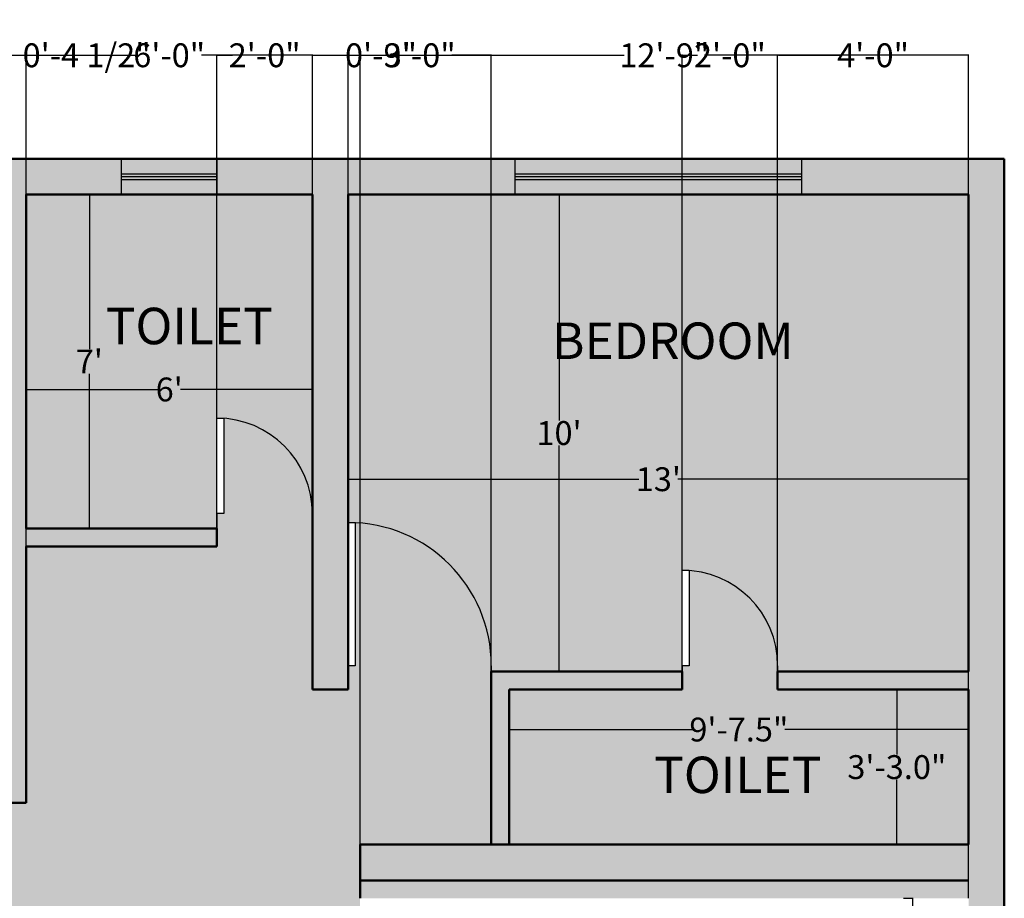
# Model space of a CAD drawing. Units: inches. Extents: x 1379 to 6665, y -118 to 1026.
# Tile 11 of 29: x 2532 to 2779, y 426 to 647. Entities that reach past the tile are written whole.
import ezdxf

# ---------------------------------------------------------------- set-up
doc = ezdxf.new("R2010")
doc.units = ezdxf.units.IN
doc.header["$MEASUREMENT"] = 0
for name, color, linetype, lineweight in [('A-ANNO-DIMS', 2, 'Continuous', 18), ('A-AREA-IDEN', 7, 'Continuous', 25), ('A-DOOR', 1, 'Continuous', 25), ('A-FLOR-PATT', 252, 'Continuous', 13), ('A-GLAZ', 2, 'Continuous', 25), ('A-WALL', 7, 'Continuous', 50), ('A-WALL-PATT', 8, 'Continuous', 13)]:
    doc.layers.add(name, color=color, linetype=linetype, lineweight=lineweight)
doc.styles.get("Standard").update_dxf_attribs({"font": 'arial.ttf'})
doc.dimstyles.get("Standard").update_dxf_attribs({"dimtxt": 6, "dimasz": 0.18, "dimexe": 0.18, "dimexo": 0.0625, "dimgap": 0.09, "dimtad": 0, "dimtih": 1, "dimtoh": 1, "dimdec": 1, "dimzin": 0, "dimdsep": 46, "dimlunit": 3, "dimtxsty": 'Standard', "dimcen": 0.09, "dimclrt": 250, "dimadec": 0, "dimazin": 0, "dimtfac": 1, "dimtdec": 1, "dimtofl": 0, "dimtmove": 0, "dimatfit": 3, "dimfxl": 1, "dimtolj": 1, "dimtzin": 0, "dimarcsym": 0})

# ---------------------------------------------------------------- blocks, each defined once
blk = doc.blocks.new('*D24')
at = {"layer": 'A-ANNO-DIMS', "color": 0, "lineweight": -2, "transparency": 16777216}
for p, q in [((2753.97, 425.93), (2756.45, 425.93)), ((2756.27, 425.75), (2756.27, 387.02)), ((2756.27, 342.11), (2756.27, 380.84)), ((2753.97, 341.93), (2756.45, 341.93))]:
    blk.add_line(p, q, dxfattribs=at)
at = {"layer": 'A-ANNO-DIMS', "color": 0, "transparency": 16777216}
for points in [[(2756.24, 425.75), (2756.3, 425.75), (2756.27, 425.93)], [(2756.24, 342.11), (2756.3, 342.11), (2756.27, 341.93)]]:
    blk.add_solid(points, dxfattribs=at)
at = {"layer": 'Defpoints', "color": 0, "transparency": 16777216}
for p in [(2753.9, 425.93), (2753.9, 341.93), (2756.27, 341.93)]:
    blk.add_point(p, dxfattribs=at)
at = {"layer": 'A-ANNO-DIMS', "color": 0, "transparency": 16777216, "insert": (2756.27, 383.93), "char_height": 6, "attachment_point": 5}
blk.add_mtext("\\A1;7'", dxfattribs=at)
blk = doc.blocks.new('*U2')
for p, q in [((0, 0), (0, -6)), ((24, 0), (24, -6))]:
    blk.add_line(p, q)
blk.add_lwpolyline([(0, 0), (0, 24), (1.75, 24), (1.75, 0)], close=True)
blk.add_arc((0, 0), 24, 0, 90)
blk = doc.blocks.new('*U3')
for p, q in [((0, 0), (0, -6)), ((36, 0), (36, -6))]:
    blk.add_line(p, q)
blk.add_lwpolyline([(0, 0), (0, 36), (1.75, 36), (1.75, 0)], close=True)
blk.add_arc((0, 0), 36, 0, 90)
blk = doc.blocks.new('*D30')
at = {"layer": 'A-ANNO-DIMS', "color": 0, "lineweight": -2, "transparency": 16777216}
for p, q in [((2533.35, 553.83), (2533.35, 553.71)), ((2533.53, 553.89), (2566.48, 553.89)), ((2605.17, 553.89), (2572.22, 553.89)), ((2605.35, 553.95), (2605.35, 554.07))]:
    blk.add_line(p, q, dxfattribs=at)
at = {"layer": 'A-ANNO-DIMS', "color": 0, "transparency": 16777216}
for points in [[(2533.53, 553.92), (2533.53, 553.86), (2533.35, 553.89)], [(2605.17, 553.92), (2605.17, 553.86), (2605.35, 553.89)]]:
    blk.add_solid(points, dxfattribs=at)
at = {"layer": 'Defpoints', "color": 0, "transparency": 16777216}
for p in [(2533.35, 553.89), (2605.35, 553.89), (2605.35, 553.89)]:
    blk.add_point(p, dxfattribs=at)
at = {"layer": 'A-ANNO-DIMS', "color": 0, "transparency": 16777216, "insert": (2569.35, 553.89), "char_height": 6, "attachment_point": 5}
blk.add_mtext("\\A1;6'", dxfattribs=at)
blk = doc.blocks.new('*D31')
at = {"layer": 'A-ANNO-DIMS', "color": 0, "lineweight": -2, "transparency": 16777216}
for p, q in [((2546.25, 602.93), (2549.44, 602.93)), ((2549.26, 602.75), (2549.26, 564.02)), ((2549.26, 519.11), (2549.26, 557.84)), ((2546.25, 518.93), (2549.44, 518.93))]:
    blk.add_line(p, q, dxfattribs=at)
at = {"layer": 'A-ANNO-DIMS', "color": 0, "transparency": 16777216}
for points in [[(2549.23, 602.75), (2549.29, 602.75), (2549.26, 602.93)], [(2549.23, 519.11), (2549.29, 519.11), (2549.26, 518.93)]]:
    blk.add_solid(points, dxfattribs=at)
at = {"layer": 'Defpoints', "color": 0, "transparency": 16777216}
for p in [(2546.19, 602.93), (2546.19, 518.93), (2549.26, 518.93)]:
    blk.add_point(p, dxfattribs=at)
at = {"layer": 'A-ANNO-DIMS', "color": 0, "transparency": 16777216, "insert": (2549.26, 560.93), "char_height": 6, "attachment_point": 5}
blk.add_mtext("\\A1;7'", dxfattribs=at)
blk = doc.blocks.new('*D32')
at = {"layer": 'A-ANNO-DIMS', "color": 0, "lineweight": -2, "transparency": 16777216}
for p, q in [((2649.05, 602.93), (2667.55, 602.93)), ((2667.37, 602.75), (2667.37, 546.09)), ((2667.37, 483.11), (2667.37, 539.78)), ((2663.46, 482.93), (2667.55, 482.93))]:
    blk.add_line(p, q, dxfattribs=at)
at = {"layer": 'A-ANNO-DIMS', "color": 0, "transparency": 16777216}
for points in [[(2667.34, 602.75), (2667.4, 602.75), (2667.37, 602.93)], [(2667.34, 483.11), (2667.4, 483.11), (2667.37, 482.93)]]:
    blk.add_solid(points, dxfattribs=at)
at = {"layer": 'Defpoints', "color": 0, "transparency": 16777216}
for p in [(2648.99, 602.93), (2663.4, 482.93), (2667.37, 482.93)]:
    blk.add_point(p, dxfattribs=at)
at = {"layer": 'A-ANNO-DIMS', "color": 0, "transparency": 16777216, "insert": (2667.37, 542.93), "char_height": 6, "attachment_point": 5}
blk.add_mtext("\\A1;10'", dxfattribs=at)
blk = doc.blocks.new('*D33')
at = {"layer": 'A-ANNO-DIMS', "color": 0, "lineweight": -2, "transparency": 16777216}
for p, q in [((2614.35, 529.56), (2614.35, 531.5)), ((2614.53, 531.32), (2687.45, 531.32)), ((2770.17, 531.32), (2697.25, 531.32)), ((2770.35, 527.24), (2770.35, 531.5))]:
    blk.add_line(p, q, dxfattribs=at)
at = {"layer": 'A-ANNO-DIMS', "color": 0, "transparency": 16777216}
for points in [[(2614.53, 531.35), (2614.53, 531.29), (2614.35, 531.32)], [(2770.17, 531.35), (2770.17, 531.29), (2770.35, 531.32)]]:
    blk.add_solid(points, dxfattribs=at)
at = {"layer": 'Defpoints', "color": 0, "transparency": 16777216}
for p in [(2770.35, 531.32), (2614.35, 529.5), (2770.35, 527.18)]:
    blk.add_point(p, dxfattribs=at)
at = {"layer": 'A-ANNO-DIMS', "color": 0, "transparency": 16777216, "insert": (2692.35, 531.32), "char_height": 6, "attachment_point": 5}
blk.add_mtext("\\A1;13'", dxfattribs=at)
blk = doc.blocks.new('*D34')
at = {"layer": 'A-ANNO-DIMS', "color": 0, "lineweight": -2, "transparency": 16777216}
for p, q in [((2751.31, 478.43), (2752.51, 478.43)), ((2752.33, 478.25), (2752.33, 462.09)), ((2752.33, 439.61), (2752.33, 455.78)), ((2751.31, 439.43), (2752.51, 439.43))]:
    blk.add_line(p, q, dxfattribs=at)
at = {"layer": 'A-ANNO-DIMS', "color": 0, "transparency": 16777216}
for points in [[(2752.3, 478.25), (2752.36, 478.25), (2752.33, 478.43)], [(2752.3, 439.61), (2752.36, 439.61), (2752.33, 439.43)]]:
    blk.add_solid(points, dxfattribs=at)
at = {"layer": 'Defpoints', "color": 0, "transparency": 16777216}
for p in [(2751.25, 478.43), (2751.25, 439.43), (2752.33, 439.43)]:
    blk.add_point(p, dxfattribs=at)
at = {"layer": 'A-ANNO-DIMS', "color": 0, "transparency": 16777216, "insert": (2752.33, 458.93), "char_height": 6, "attachment_point": 5}
blk.add_mtext('\\A1;3\'-3.0"', dxfattribs=at)
blk = doc.blocks.new('*D35')
at = {"layer": 'A-ANNO-DIMS', "color": 0, "lineweight": -2, "transparency": 16777216}
for p, q in [((2654.85, 463.04), (2654.85, 468.56)), ((2655.03, 468.38), (2701.04, 468.38)), ((2770.17, 468.38), (2724.16, 468.38)), ((2770.35, 459), (2770.35, 468.56))]:
    blk.add_line(p, q, dxfattribs=at)
at = {"layer": 'A-ANNO-DIMS', "color": 0, "transparency": 16777216}
for points in [[(2655.03, 468.41), (2655.03, 468.35), (2654.85, 468.38)], [(2770.17, 468.41), (2770.17, 468.35), (2770.35, 468.38)]]:
    blk.add_solid(points, dxfattribs=at)
at = {"layer": 'Defpoints', "color": 0, "transparency": 16777216}
for p in [(2770.35, 468.38), (2654.85, 462.97), (2770.35, 458.93)]:
    blk.add_point(p, dxfattribs=at)
at = {"layer": 'A-ANNO-DIMS', "color": 0, "transparency": 16777216, "insert": (2712.6, 468.38), "char_height": 6, "attachment_point": 5}
blk.add_mtext('\\A1;9\'-7.5"', dxfattribs=at)
blk = doc.blocks.new('WIN-1800')
for p, q in [((0, 0.73), (72, 0.73)), ((0, 0), (72, 0))]:
    blk.add_line(p, q)
blk = doc.blocks.new('WIN-600')
for p, q in [((0, 24), (0, 0)), ((0.73, 24), (0.73, 0))]:
    blk.add_line(p, q)
blk = doc.blocks.new('*D155')
at = {"layer": 'A-ANNO-DIMS', "color": 0, "lineweight": -2, "transparency": 16777216}
for p, q in [((2528.85, 603), (2528.85, 638.11)), ((2529.03, 637.93), (2533.17, 637.93)), ((2533.35, 603), (2533.35, 638.11)), ((2533.35, 637.93), (2533.53, 637.93))]:
    blk.add_line(p, q, dxfattribs=at)
at = {"layer": 'A-ANNO-DIMS', "color": 0, "transparency": 16777216}
for points in [[(2529.03, 637.96), (2529.03, 637.9), (2528.85, 637.93)], [(2533.17, 637.96), (2533.17, 637.9), (2533.35, 637.93)]]:
    blk.add_solid(points, dxfattribs=at)
at = {"layer": 'Defpoints', "color": 0, "transparency": 16777216}
for p in [(2533.35, 637.93), (2528.85, 602.93), (2533.35, 602.93)]:
    blk.add_point(p, dxfattribs=at)
at = {"layer": 'A-ANNO-DIMS', "color": 250, "transparency": 16777216, "insert": (2548.59, 637.93), "char_height": 6, "attachment_point": 5}
blk.add_mtext('\\A1;0\'-4 1/2"', dxfattribs=at)
blk = doc.blocks.new('*D156')
at = {"layer": 'A-ANNO-DIMS', "color": 0, "lineweight": -2, "transparency": 16777216}
for p, q in [((2605.35, 603), (2605.35, 638.11)), ((2605.53, 637.93), (2614.17, 637.93)), ((2614.35, 603), (2614.35, 638.11)), ((2614.35, 637.93), (2614.53, 637.93))]:
    blk.add_line(p, q, dxfattribs=at)
at = {"layer": 'A-ANNO-DIMS', "color": 0, "transparency": 16777216}
for points in [[(2605.53, 637.96), (2605.53, 637.9), (2605.35, 637.93)], [(2614.17, 637.96), (2614.17, 637.9), (2614.35, 637.93)]]:
    blk.add_solid(points, dxfattribs=at)
at = {"layer": 'Defpoints', "color": 0, "transparency": 16777216}
for p in [(2614.35, 637.93), (2605.35, 602.93), (2614.35, 602.93)]:
    blk.add_point(p, dxfattribs=at)
at = {"layer": 'A-ANNO-DIMS', "color": 250, "transparency": 16777216, "insert": (2622.6, 637.93), "char_height": 6, "attachment_point": 5}
blk.add_mtext('\\A1;0\'-9"', dxfattribs=at)
blk = doc.blocks.new('*D157')
at = {"layer": 'A-ANNO-DIMS', "color": 0, "lineweight": -2, "transparency": 16777216}
for p, q in [((2533.35, 514.5), (2533.35, 638.11)), ((2533.53, 637.93), (2561.27, 637.93)), ((2605.17, 637.93), (2577.43, 637.93)), ((2605.35, 478.5), (2605.35, 638.11))]:
    blk.add_line(p, q, dxfattribs=at)
at = {"layer": 'A-ANNO-DIMS', "color": 0, "transparency": 16777216}
for points in [[(2533.53, 637.96), (2533.53, 637.9), (2533.35, 637.93)], [(2605.17, 637.96), (2605.17, 637.9), (2605.35, 637.93)]]:
    blk.add_solid(points, dxfattribs=at)
at = {"layer": 'Defpoints', "color": 0, "transparency": 16777216}
for p in [(2605.35, 637.93), (2533.35, 514.43), (2605.35, 478.43)]:
    blk.add_point(p, dxfattribs=at)
at = {"layer": 'A-ANNO-DIMS', "color": 250, "transparency": 16777216, "insert": (2569.35, 637.93), "char_height": 6, "attachment_point": 5}
blk.add_mtext('\\A1;6\'-0"', dxfattribs=at)
blk = doc.blocks.new('*D158')
at = {"layer": 'A-ANNO-DIMS', "color": 0, "lineweight": -2, "transparency": 16777216}
for p, q in [((2617.35, 426), (2617.35, 638.11)), ((2617.53, 637.93), (2683.74, 637.93)), ((2770.17, 637.93), (2703.96, 637.93)), ((2770.35, 426), (2770.35, 638.11))]:
    blk.add_line(p, q, dxfattribs=at)
at = {"layer": 'A-ANNO-DIMS', "color": 0, "transparency": 16777216}
for points in [[(2617.53, 637.96), (2617.53, 637.9), (2617.35, 637.93)], [(2770.17, 637.96), (2770.17, 637.9), (2770.35, 637.93)]]:
    blk.add_solid(points, dxfattribs=at)
at = {"layer": 'Defpoints', "color": 0, "transparency": 16777216}
for p in [(2770.35, 637.93), (2617.35, 425.93), (2770.35, 425.93)]:
    blk.add_point(p, dxfattribs=at)
at = {"layer": 'A-ANNO-DIMS', "color": 250, "transparency": 16777216, "insert": (2693.85, 637.93), "char_height": 6, "attachment_point": 5}
blk.add_mtext('\\A1;12\'-9"', dxfattribs=at)
blk = doc.blocks.new('*D162')
at = {"layer": 'A-ANNO-DIMS', "color": 0, "lineweight": -2, "transparency": 16777216}
for p, q in [((2581.35, 519), (2581.35, 638.11)), ((2581.53, 637.93), (2585.23, 637.93)), ((2605.17, 637.93), (2601.47, 637.93)), ((2605.35, 519), (2605.35, 638.11))]:
    blk.add_line(p, q, dxfattribs=at)
at = {"layer": 'A-ANNO-DIMS', "color": 0, "transparency": 16777216}
for points in [[(2581.53, 637.96), (2581.53, 637.9), (2581.35, 637.93)], [(2605.17, 637.96), (2605.17, 637.9), (2605.35, 637.93)]]:
    blk.add_solid(points, dxfattribs=at)
at = {"layer": 'Defpoints', "color": 0, "transparency": 16777216}
for p in [(2605.35, 637.93), (2581.35, 518.93), (2605.35, 518.93)]:
    blk.add_point(p, dxfattribs=at)
at = {"layer": 'A-ANNO-DIMS', "color": 250, "transparency": 16777216, "insert": (2593.35, 637.93), "char_height": 6, "attachment_point": 5}
blk.add_mtext('\\A1;2\'-0"', dxfattribs=at)
blk = doc.blocks.new('*D164')
at = {"layer": 'A-ANNO-DIMS', "color": 0, "lineweight": -2, "transparency": 16777216}
for p, q in [((2614.35, 483), (2614.35, 638.11)), ((2614.53, 637.93), (2624.29, 637.93)), ((2650.17, 637.93), (2640.41, 637.93)), ((2650.35, 483), (2650.35, 638.11))]:
    blk.add_line(p, q, dxfattribs=at)
at = {"layer": 'A-ANNO-DIMS', "color": 0, "transparency": 16777216}
for points in [[(2614.53, 637.96), (2614.53, 637.9), (2614.35, 637.93)], [(2650.17, 637.96), (2650.17, 637.9), (2650.35, 637.93)]]:
    blk.add_solid(points, dxfattribs=at)
at = {"layer": 'Defpoints', "color": 0, "transparency": 16777216}
for p in [(2650.35, 637.93), (2614.35, 482.93), (2650.35, 482.93)]:
    blk.add_point(p, dxfattribs=at)
at = {"layer": 'A-ANNO-DIMS', "color": 250, "transparency": 16777216, "insert": (2632.35, 637.93), "char_height": 6, "attachment_point": 5}
blk.add_mtext('\\A1;3\'-0"', dxfattribs=at)
blk = doc.blocks.new('*D166')
at = {"layer": 'A-ANNO-DIMS', "color": 0, "lineweight": -2, "transparency": 16777216}
for p, q in [((2698.35, 483), (2698.35, 638.11)), ((2698.53, 637.93), (2702.23, 637.93)), ((2722.17, 637.93), (2718.47, 637.93)), ((2722.35, 483), (2722.35, 638.11))]:
    blk.add_line(p, q, dxfattribs=at)
at = {"layer": 'A-ANNO-DIMS', "color": 0, "transparency": 16777216}
for points in [[(2698.53, 637.96), (2698.53, 637.9), (2698.35, 637.93)], [(2722.17, 637.96), (2722.17, 637.9), (2722.35, 637.93)]]:
    blk.add_solid(points, dxfattribs=at)
at = {"layer": 'Defpoints', "color": 0, "transparency": 16777216}
for p in [(2722.35, 637.93), (2698.35, 482.93), (2722.35, 482.93)]:
    blk.add_point(p, dxfattribs=at)
at = {"layer": 'A-ANNO-DIMS', "color": 250, "transparency": 16777216, "insert": (2710.35, 637.93), "char_height": 6, "attachment_point": 5}
blk.add_mtext('\\A1;2\'-0"', dxfattribs=at)
blk = doc.blocks.new('*D167')
at = {"layer": 'A-ANNO-DIMS', "color": 0, "lineweight": -2, "transparency": 16777216}
for p, q in [((2722.35, 483), (2722.35, 638.11)), ((2722.53, 637.93), (2738.16, 637.93)), ((2770.17, 637.93), (2754.54, 637.93)), ((2770.35, 483), (2770.35, 638.11))]:
    blk.add_line(p, q, dxfattribs=at)
at = {"layer": 'A-ANNO-DIMS', "color": 0, "transparency": 16777216}
for points in [[(2722.53, 637.96), (2722.53, 637.9), (2722.35, 637.93)], [(2770.17, 637.96), (2770.17, 637.9), (2770.35, 637.93)]]:
    blk.add_solid(points, dxfattribs=at)
at = {"layer": 'Defpoints', "color": 0, "transparency": 16777216}
for p in [(2770.35, 637.93), (2722.35, 482.93), (2770.35, 482.93)]:
    blk.add_point(p, dxfattribs=at)
at = {"layer": 'A-ANNO-DIMS', "color": 250, "transparency": 16777216, "insert": (2746.35, 637.93), "char_height": 6, "attachment_point": 5}
blk.add_mtext('\\A1;4\'-0"', dxfattribs=at)

msp = doc.modelspace()

# ---------------------------------------------------------------- hatches: boundary and pattern name
at = {"layer": 'A-FLOR-PATT', "transparency": 33554590}
h = msp.add_hatch(color=256, dxfattribs=at)
h.dxf.hatch_style = 1
h.paths.add_polyline_path([(2290.35, 490.43), (2290.35, 602.93), (2369.85, 602.93), (2369.85, 611.93), (2281.35, 611.93), (2281.35, 499.43), (2281.35, 431.93), (2290.35, 431.93), (2290.35, 449.93), (2462.85, 449.93), (2462.85, 458.93), (2290.35, 458.93)])
h.paths.add_polyline_path([(2462.85, 341.93), (2290.35, 341.93), (2290.35, 359.93), (2281.35, 359.93), (2281.35, 179.93), (2359.96, 179.93), (2359.96, 188.93), (2290.35, 188.93), (2290.35, 332.93), (2462.85, 332.93)])
h.paths.add_polyline_path([(2557.35, 188.93), (2533.35, 188.93), (2533.35, 272.93), (2581.35, 272.93), (2581.35, 277.43), (2533.35, 277.43), (2533.35, 332.93), (2533.35, 341.93), (2498.82, 341.93), (2498.85, 332.93), (2528.85, 332.93), (2528.85, 188.93), (2431.96, 188.93), (2431.96, 179.93), (2557.35, 179.93)])
h.paths.add_polyline_path([(2666.85, 188.93), (2614.35, 188.93), (2614.35, 277.43), (2605.35, 277.43), (2605.35, 272.93), (2605.35, 188.93), (2581.35, 188.93), (2581.35, 179.93), (2617.35, 179.93), (2666.85, 179.93)])
h.paths.add_polyline_path([(2779.35, 296.93), (2770.35, 296.93), (2770.35, 284.93), (2740.35, 284.93), (2740.35, 280.43), (2770.35, 280.43), (2770.35, 188.93), (2738.85, 188.93), (2738.85, 179.93), (2779.35, 179.93)])
h.paths.add_polyline_path([(2779.35, 611.93), (2728.35, 611.93), (2728.35, 602.93), (2770.35, 602.93), (2770.35, 482.93), (2722.35, 482.93), (2722.35, 478.43), (2770.35, 478.43), (2770.35, 439.43), (2626.35, 439.43), (2617.35, 439.43), (2617.35, 430.43), (2617.35, 425.93), (2770.35, 425.93), (2770.35, 341.93), (2617.35, 341.93), (2569.35, 341.93), (2569.35, 332.93), (2617.35, 332.93), (2681.85, 332.93), (2681.85, 284.93), (2654.35, 284.93), (2654.35, 280.43), (2681.85, 280.43), (2716.35, 280.43), (2716.35, 284.93), (2686.35, 284.93), (2686.35, 332.93), (2770.35, 332.93), (2770.35, 320.93), (2779.35, 320.93)])
h.paths.add_polyline_path([(2698.35, 482.93), (2650.35, 482.93), (2650.35, 478.43), (2650.35, 439.43), (2654.85, 439.43), (2654.85, 478.43), (2698.35, 478.43)], flags=17)
h.paths.add_polyline_path([(2614.35, 602.93), (2656.35, 602.93), (2656.35, 611.93), (2581.35, 611.93), (2581.35, 602.93), (2605.35, 602.93), (2605.35, 478.43), (2614.35, 478.43), (2614.35, 482.93)], flags=17)
h.paths.add_polyline_path([(2557.35, 611.93), (2521.35, 611.93), (2441.85, 611.93), (2441.85, 602.93), (2521.35, 602.93), (2528.85, 602.93), (2528.85, 458.93), (2498.73, 458.93), (2498.85, 449.93), (2533.35, 449.93), (2533.35, 514.43), (2581.35, 514.43), (2581.35, 518.93), (2533.35, 518.93), (2533.35, 602.93), (2557.35, 602.93)])
at = {"layer": 'A-WALL-PATT', "transparency": 33554590}
h = msp.add_hatch(color=256, dxfattribs=at)
h.dxf.hatch_style = 1
h.paths.add_polyline_path([(2581.35, 611.93), (2557.35, 611.93), (2557.35, 608.17), (2581.35, 608.17)])
h.paths.add_polyline_path([(2581.35, 606.7), (2557.35, 606.7), (2557.35, 602.93), (2581.35, 602.93)])
h.paths.add_polyline_path([(2581.35, 607.43), (2557.35, 607.43), (2557.35, 606.7), (2581.35, 606.7)])
h.paths.add_polyline_path([(2581.35, 608.17), (2557.35, 608.17), (2557.35, 607.43), (2581.35, 607.43)])
at = {"layer": 'A-WALL-PATT', "transparency": 33554564}
h = msp.add_hatch(color=256, dxfattribs=at)
h.dxf.hatch_style = 1
h.paths.add_polyline_path([(2728.35, 611.93), (2656.35, 611.93), (2656.35, 608.17), (2728.35, 608.17)])
h.paths.add_polyline_path([(2728.35, 607.43), (2656.35, 607.43), (2656.35, 606.7), (2728.35, 606.7)])
h.paths.add_polyline_path([(2728.35, 608.17), (2656.35, 608.17), (2656.35, 607.43), (2728.35, 607.43)])
h.paths.add_polyline_path([(2728.35, 606.7), (2656.35, 606.7), (2656.35, 602.93), (2728.35, 602.93)])
at = {"layer": 'A-WALL-PATT', "transparency": 33554590}
h = msp.add_hatch(color=256, dxfattribs=at)
h.dxf.hatch_style = 1
h.paths.add_polyline_path([(2528.85, 602.93), (2290.35, 602.93), (2290.35, 490.43), (2290.35, 458.93), (2462.85, 458.93), (2462.85, 491.93), (2464.6, 491.93), (2464.6, 491.89, -0.376042), (2498.73, 458.93), (2528.85, 458.93)])
h.paths.add_polyline_path([(2617.35, 425.93), (2617.35, 430.43), (2617.35, 439.43), (2626.35, 439.43), (2650.35, 439.43), (2650.35, 478.43), (2650.35, 484.43, 0.400041), (2616.1, 520.39), (2616.1, 484.43), (2614.35, 484.43), (2614.35, 478.43), (2605.35, 478.43), (2605.35, 522.68, 0.392996), (2583.1, 546.62), (2583.1, 522.68), (2581.35, 522.68), (2581.35, 516.68), (2581.35, 514.43), (2533.35, 514.43), (2533.35, 449.93), (2498.85, 449.93), (2498.73, 458.93, 0.376042), (2464.6, 491.89), (2464.6, 455.93), (2462.85, 455.93), (2462.85, 449.93), (2290.35, 449.93), (2290.35, 341.93), (2462.85, 341.93), (2462.85, 374.93), (2464.6, 374.93), (2464.6, 374.89, -0.376042), (2498.73, 341.93), (2533.35, 341.93), (2533.35, 332.93), (2533.35, 277.43), (2581.35, 277.43), (2581.35, 281.18), (2581.35, 305.18), (2583.1, 305.18), (2583.1, 305.12, -0.392996), (2605.35, 281.18), (2605.35, 277.43), (2614.35, 277.43), (2614.35, 283.43), (2614.35, 323.43), (2616.1, 323.43), (2616.1, 323.4, -0.390605), (2654.32, 284.93), (2681.85, 284.93), (2681.85, 332.93), (2614.35, 332.93), (2569.35, 332.93), (2569.35, 341.93), (2617.35, 341.93), (2617.35, 383.93)])
h.paths.add_polyline_path([(2605.35, 602.93), (2533.35, 602.93), (2533.35, 518.93), (2581.35, 518.93), (2581.35, 522.68), (2581.35, 546.68), (2583.1, 546.68), (2583.1, 546.62, -0.392996), (2605.35, 522.68)])
h.paths.add_polyline_path([(2770.35, 602.93), (2614.35, 602.93), (2614.35, 520.43), (2616.1, 520.43), (2616.1, 520.39, -0.400041), (2650.35, 484.43), (2650.35, 482.93), (2698.35, 482.93), (2698.35, 484.43), (2698.35, 508.43), (2700.1, 508.43), (2700.1, 508.37, -0.392996), (2722.35, 484.43), (2722.35, 482.93), (2770.35, 482.93)])
h.paths.add_polyline_path([(2528.85, 332.93), (2498.85, 332.93), (2498.82, 341.93), (2498.73, 341.93, 0.376042), (2464.6, 374.89), (2464.6, 374.93), (2462.85, 374.93), (2462.85, 341.93), (2462.85, 332.93), (2290.35, 332.93), (2290.35, 188.93), (2528.85, 188.93)])
h.paths.add_polyline_path([(2605.35, 272.93), (2605.35, 277.43), (2605.35, 281.18, 0.392996), (2583.1, 305.12), (2583.1, 281.18), (2581.35, 281.18), (2581.35, 277.43), (2581.35, 275.18), (2581.35, 272.93), (2533.35, 272.93), (2533.35, 188.93), (2605.35, 188.93)])
h.paths.add_polyline_path([(2770.35, 280.43), (2740.35, 280.43), (2740.35, 286.43, 0.392996), (2718.1, 310.37), (2718.1, 286.43), (2716.35, 286.43), (2716.35, 280.43), (2681.85, 280.43), (2654.35, 280.43), (2654.35, 283.43, 0.401453), (2616.1, 323.4), (2616.1, 283.43), (2614.35, 283.43), (2614.35, 277.43), (2614.35, 188.93), (2617.35, 188.93), (2770.35, 188.93)])
h.paths.add_polyline_path([(2770.35, 332.93), (2686.35, 332.93), (2686.35, 284.93), (2716.35, 284.93), (2716.35, 286.43), (2716.35, 310.43), (2718.1, 310.43), (2718.1, 310.37, -0.392996), (2740.35, 286.43), (2740.35, 284.93), (2770.35, 284.93)])
h.paths.add_polyline_path([(2770.35, 478.43), (2722.35, 478.43), (2722.35, 484.43, 0.392996), (2700.1, 508.37), (2700.1, 484.43), (2698.35, 484.43), (2698.35, 482.93), (2698.35, 478.43), (2654.85, 478.43), (2654.85, 439.43), (2770.35, 439.43)])
h.paths.add_polyline_path([(2372.98, 539.34), (2443.91, 539.34), (2443.91, 553.57), (2372.98, 553.57)], flags=24)
h.paths.add_polyline_path([(2370.72, 389.31), (2479.4, 389.31), (2479.4, 403.55), (2370.72, 403.55)], flags=24)
h.paths.add_polyline_path([(2550.99, 562.74), (2600.58, 562.74), (2600.58, 576.98), (2550.99, 576.98)], flags=24)
h.paths.add_polyline_path([(2663.19, 559.03), (2734.13, 559.03), (2734.13, 573.27), (2663.19, 573.27)], flags=24)
h.paths.add_polyline_path([(2372.98, 254.81), (2443.91, 254.81), (2443.91, 269.04), (2372.98, 269.04)], flags=24)
h.paths.add_polyline_path([(2545.25, 230.45), (2594.84, 230.45), (2594.84, 244.68), (2545.25, 244.68)], flags=24)
h.paths.add_polyline_path([(2664.48, 230.74), (2735.42, 230.74), (2735.42, 244.97), (2664.48, 244.97)], flags=24)
h.paths.add_polyline_path([(2704.72, 315.06), (2754.31, 315.06), (2754.31, 329.29), (2704.72, 329.29)], flags=24)
h.paths.add_polyline_path([(2688.89, 449.86), (2738.48, 449.86), (2738.48, 464.09), (2688.89, 464.09)], flags=24)

# ---------------------------------------------------------------- linework, layer by layer
at = {"layer": 'A-GLAZ'}
for p, q in [((2557.35, 606.7), (2581.35, 606.7)), ((2656.35, 606.7), (2728.35, 606.7))]:
    msp.add_line(p, q, dxfattribs=at)
for points in [[(2557.35, 611.93), (2581.35, 611.93), (2581.35, 602.93), (2557.35, 602.93)], [(2656.35, 611.93), (2728.35, 611.93), (2728.35, 602.93), (2656.35, 602.93)]]:
    msp.add_lwpolyline(points, close=True, dxfattribs=at)
at = {"layer": 'A-WALL'}
for p, q in [((2779.35, 611.93), (2521.35, 611.93)), ((2779.35, 611.93), (2779.35, 179.93)), ((2533.35, 518.93), (2533.35, 602.93)), ((2605.35, 602.93), (2533.35, 602.93)), ((2605.35, 478.43), (2605.35, 602.93)), ((2770.35, 602.93), (2614.35, 602.93)), ((2614.35, 482.93), (2614.35, 602.93)), ((2770.35, 602.93), (2770.35, 482.93)), ((2581.35, 518.93), (2533.35, 518.93)), ((2581.35, 518.93), (2581.35, 514.43)), ((2605.35, 518.93), (2605.35, 514.43)), ((2533.35, 449.93), (2533.35, 514.43)), ((2581.35, 514.43), (2533.35, 514.43)), ((2614.35, 482.93), (2614.35, 478.43)), ((2698.35, 482.93), (2650.35, 482.93)), ((2650.35, 482.93), (2650.35, 478.43)), ((2698.35, 478.43), (2698.35, 482.93)), ((2770.35, 482.93), (2722.35, 482.93)), ((2722.35, 478.43), (2722.35, 482.93)), ((2614.35, 478.43), (2605.35, 478.43)), ((2650.35, 478.43), (2650.35, 439.43)), ((2698.35, 478.43), (2654.85, 478.43)), ((2654.85, 478.43), (2654.85, 439.43)), ((2770.35, 478.43), (2722.35, 478.43)), ((2770.35, 478.43), (2770.35, 439.43)), ((2533.35, 449.93), (2498.85, 449.93)), ((2617.35, 430.43), (2617.35, 439.43)), ((2617.35, 439.43), (2626.35, 439.43)), ((2626.35, 439.43), (2770.35, 439.43)), ((2617.35, 430.43), (2617.35, 425.93)), ((2626.35, 430.43), (2617.35, 430.43)), ((2626.35, 430.43), (2770.35, 430.43))]:
    msp.add_line(p, q, dxfattribs=at)

# ---------------------------------------------------------------- block references
at = {"layer": 'A-DOOR'}
for name, p in [('*U2', (2581.35, 522.68)), ('*U3', (2614.35, 484.43)), ('*U2', (2698.35, 484.43))]:
    msp.add_blockref(name, p, dxfattribs=at)
at = {"layer": 'A-GLAZ', "rotation": 90.00000000000163}
msp.add_blockref('WIN-600', (2581.35, 607.43), dxfattribs=at)
at = {"layer": 'A-GLAZ'}
msp.add_blockref('WIN-1800', (2656.35, 607.43), dxfattribs=at)

# ---------------------------------------------------------------- texts
at = {"layer": 'A-AREA-IDEN'}
for s, p in [('TOILET', (2553.36, 565.27)), ('BEDROOM', (2665.56, 561.56)), ('TOILET', (2691.27, 452.39))]:
    msp.add_text(s, height=9.17, dxfattribs=at).set_placement(p)

# ---------------------------------------------------------------- dimensions: what is measured, and where the dimension line sits
at = {"layer": 'A-ANNO-DIMS'}
for base, p1, p2, override, picture, middle in [((2533.35, 637.93), (2528.85, 602.93), (2533.35, 602.93), {"dimdec": 1, "dimlfac": 1, "dimrnd": 0, "dimzin": 1, "dimdsep": 46, "dimlunit": 4, "dimfrac": 2}, '*D155', (2548.59, 637.93)), ((2605.35, 637.93), (2533.35, 514.43), (2605.35, 478.43), {"dimdec": 1, "dimlfac": 1, "dimrnd": 0, "dimzin": 1, "dimdsep": 46, "dimlunit": 4, "dimfrac": 2}, '*D157', (2569.35, 637.93)), ((2605.35, 637.93), (2581.35, 518.93), (2605.35, 518.93), {"dimdec": 1, "dimlfac": 1, "dimrnd": 0, "dimzin": 1, "dimdsep": 46, "dimlunit": 4, "dimfrac": 2}, '*D162', (2593.35, 637.93)), ((2614.35, 637.93), (2605.35, 602.93), (2614.35, 602.93), {"dimdec": 1, "dimlfac": 1, "dimrnd": 0, "dimzin": 1, "dimdsep": 46, "dimlunit": 4, "dimfrac": 2}, '*D156', (2622.6, 637.93)), ((2650.35, 637.93), (2614.35, 482.93), (2650.35, 482.93), {"dimdec": 1, "dimlfac": 1, "dimrnd": 0, "dimzin": 1, "dimdsep": 46, "dimlunit": 4, "dimfrac": 2}, '*D164', (2632.35, 637.93)), ((2770.35, 637.93), (2617.35, 425.93), (2770.35, 425.93), {"dimdec": 1, "dimlfac": 1, "dimrnd": 0, "dimzin": 1, "dimdsep": 46, "dimlunit": 4, "dimfrac": 2}, '*D158', (2693.85, 637.93)), ((2722.35, 637.93), (2698.35, 482.93), (2722.35, 482.93), {"dimdec": 1, "dimlfac": 1, "dimrnd": 0, "dimzin": 1, "dimdsep": 46, "dimlunit": 4, "dimfrac": 2}, '*D166', (2710.35, 637.93)), ((2770.35, 637.93), (2722.35, 482.93), (2770.35, 482.93), {"dimdec": 1, "dimlfac": 1, "dimrnd": 0, "dimzin": 1, "dimdsep": 46, "dimlunit": 4, "dimfrac": 2}, '*D167', (2746.35, 637.93)), ((2605.35, 553.89), (2533.35, 553.89), (2605.35, 553.89), {"dimclrd": 0, "dimclre": 0, "dimclrt": 0}, '*D30', (2569.35, 553.89)), ((2770.35, 531.32), (2614.35, 529.5), (2770.35, 527.18), {"dimclrd": 0, "dimclre": 0, "dimclrt": 0}, '*D33', (2692.35, 531.32)), ((2770.35, 468.38), (2654.85, 462.97), (2770.35, 458.93), {"dimclrd": 0, "dimclre": 0, "dimclrt": 0}, '*D35', (2712.6, 468.38))]:
    dim = msp.add_linear_dim(base=base, p1=p1, p2=p2, dimstyle='Standard', override=override, dxfattribs=at)
    dim.commit()
    dim.dimension.update_dxf_attribs({"geometry": picture, "text_midpoint": middle})
for base, p1, p2, picture, middle in [((2549.26, 518.93), (2546.19, 602.93), (2546.19, 518.93), '*D31', (2549.26, 560.93)), ((2667.37, 482.93), (2648.99, 602.93), (2663.4, 482.93), '*D32', (2667.37, 542.93)), ((2752.33, 439.43), (2751.25, 478.43), (2751.25, 439.43), '*D34', (2752.33, 458.93)), ((2756.27, 341.93), (2753.9, 425.93), (2753.9, 341.93), '*D24', (2756.27, 383.93))]:
    dim = msp.add_linear_dim(base=base, p1=p1, p2=p2, angle=90, dimstyle='Standard', override={"dimclrd": 0, "dimclre": 0, "dimclrt": 0}, dxfattribs=at)
    dim.commit()
    dim.dimension.update_dxf_attribs({"geometry": picture, "text_midpoint": middle})

doc.saveas('drawing.dxf')
